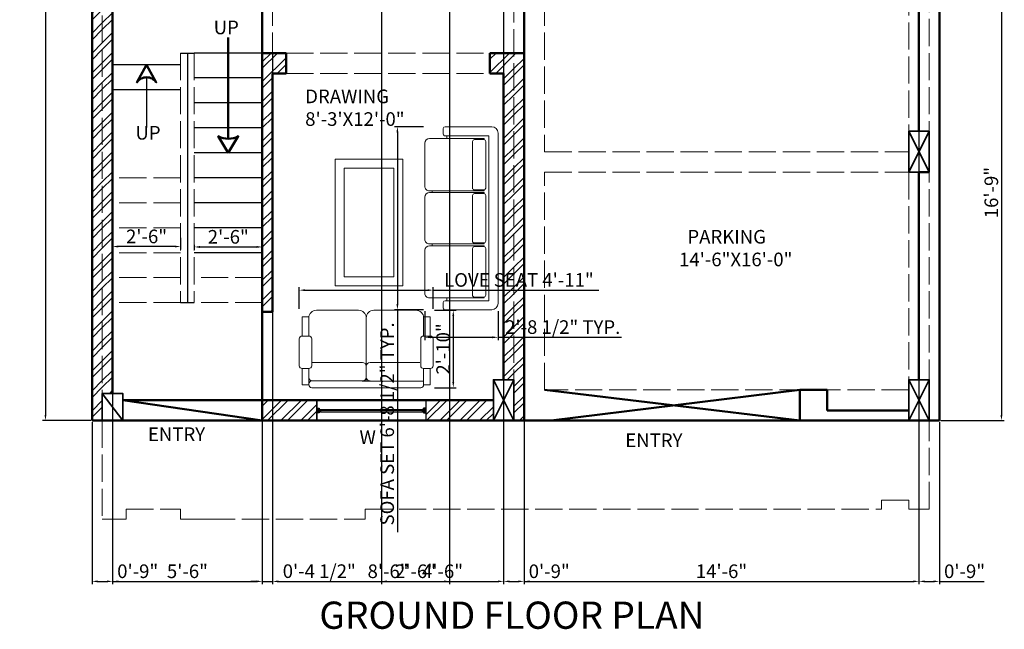
# Model space of a CAD drawing. Units: millimetres. Extents: x 4237 to 5109, y 21391 to 22486.
# Tile 6 of 17: x 4240 to 4674, y 21941 to 22209. Entities that reach past the tile are written whole.
import ezdxf

# ---------------------------------------------------------------- set-up
doc = ezdxf.new("R2010")
doc.units = ezdxf.units.MM
doc.linetypes.add('ACAD_ISO02W100', pattern=[15, 12, -3])
for name, color, linetype, lineweight in [('A-ANNO-DIMS', 2, 'Continuous', 18), ('A-ANNO-TEXT', 7, 'Continuous', 18), ('A-AREA-IDEN', 3, 'Continuous', 18), ('A-FLOR-OVHD', 1, 'ACAD_ISO02W100', 18), ('A-FLOR-STRS', 7, 'Continuous', 25), ('A-FURN', 8, 'Continuous', 18), ('A-WALL', 7, 'Continuous', 50), ('A-WALL-PATT', 252, 'Continuous', 13), ('column', 102, 'Continuous', 35), ('windows', 140, 'Continuous', 25)]:
    doc.layers.add(name, color=color, linetype=linetype, lineweight=lineweight)
doc.styles.get("Standard").update_dxf_attribs({"font": 'arial.ttf'})
doc.dimstyles.new('ISO-25', dxfattribs={"dimtxt": 6, "dimasz": 2.5, "dimexe": 1.25, "dimexo": 0.625, "dimtad": 1, "dimdec": 1, "dimlunit": 4, "dimtxsty": 'Standard', "dimcen": 2.5, "dimadec": 0, "dimazin": 0, "dimtfac": 1, "dimtdec": 1, "dimtmove": 0, "dimatfit": 3, "dimfxl": 1, "dimarcsym": 0})

# ---------------------------------------------------------------- blocks, each defined once
blk = doc.blocks.new('A$C06FC73D7')
for p, q in [((1.93, 0.8), (0.07, 0.8)), ((0, 0.73), (0, 0.22)), ((0.1, 0.22), (0.1, 0.7)), ((0.1, 0.7), (1.9, 0.7)), ((0.13, 0.648), (0.13, 0.05)), ((0.14, 0.648), (0.13, 0.648)), ((0.67, 0.664), (0.16, 0.664)), ((0.7, 0.648), (0.69, 0.648)), ((0.7, 0.05), (0.7, 0.648)), ((0.72, 0.05), (0.72, 0.648)), ((0.73, 0.648), (0.72, 0.648)), ((1.25, 0.664), (0.75, 0.664)), ((1.28, 0.648), (1.27, 0.648)), ((1.28, 0.05), (1.28, 0.648)), ((1.3, 0.05), (1.3, 0.648)), ((1.31, 0.648), (1.3, 0.648)), ((1.84, 0.664), (1.33, 0.664)), ((1.87, 0.648), (1.86, 0.648)), ((1.87, 0.05), (1.87, 0.648)), ((1.9, 0.7), (1.9, 0.22)), ((2, 0.22), (2, 0.73)), ((0.14, 0.54), (0.14, 0.644)), ((0.69, 0.54), (0.69, 0.644)), ((0.73, 0.54), (0.73, 0.644)), ((1.27, 0.54), (1.27, 0.644)), ((1.31, 0.54), (1.31, 0.644)), ((1.86, 0.54), (1.86, 0.644)), ((0.67, 0.52), (0.16, 0.52)), ((1.25, 0.52), (0.75, 0.52)), ((1.84, 0.52), (1.33, 0.52)), ((0.13, 0.24), (0.1, 0.24)), ((1.9, 0.24), (1.87, 0.24)), ((0.02, 0.2), (0.08, 0.2)), ((1.92, 0.2), (1.98, 0.2)), ((0.65, 0), (0.18, 0)), ((0.72, 0.08), (0.7, 0.08)), ((1.23, 0), (0.77, 0)), ((1.3, 0.08), (1.28, 0.08)), ((1.82, 0), (1.35, 0))]:
    blk.add_line(p, q)
for centre, radius, start, end in [((0.07, 0.73), 0.07, 90, 180), ((1.93, 0.73), 0.07, 0, 90), ((0.16, 0.644), 0.02, 90, 180), ((0.67, 0.644), 0.02, 0, 90), ((0.75, 0.644), 0.02, 90, 180), ((1.25, 0.644), 0.02, 0, 90), ((1.33, 0.644), 0.02, 90, 180), ((1.84, 0.644), 0.02, 0, 90), ((0.16, 0.54), 0.02, 180, 270), ((0.67, 0.54), 0.02, 270, 0), ((0.75, 0.54), 0.02, 180, 270), ((1.25, 0.54), 0.02, 270, 0), ((1.33, 0.54), 0.02, 180, 270), ((1.84, 0.54), 0.02, 270, 0), ((0.02, 0.22), 0.02, 180, 270), ((0.08, 0.22), 0.02, 270, 0), ((1.92, 0.22), 0.02, 180, 270), ((1.98, 0.22), 0.02, 270, 0), ((0.18, 0.05), 0.05, 180, 270), ((0.65, 0.05), 0.05, 270, 0), ((0.77, 0.05), 0.05, 180, 270), ((1.23, 0.05), 0.05, 270, 0), ((1.35, 0.05), 0.05, 180, 270), ((1.82, 0.05), 0.05, 270, 0)]:
    blk.add_arc(centre, radius, start, end)
blk = doc.blocks.new('F20')
for p, q in [((-0.558, 0.019), (0.582, 0.019)), ((-0.658, -0.181), (-0.658, -0.011)), ((-0.658, -0.011), (-0.588, -0.011)), ((-0.588, -0.011), (-0.588, -0.021)), ((-0.588, -0.091), (-0.588, -0.011)), ((-0.588, -0.181), (-0.588, -0.091)), ((-0.028, -0.051), (-0.548, -0.051)), ((-0.029, -0.05), (0.06, -0.05)), ((0.012, -0.606), (0.012, -0.051)), ((0.012, -0.205), (0.012, -0.091)), ((0.06, -0.05), (0.612, -0.05)), ((0.612, -0.181), (0.612, -0.01)), ((0.612, -0.011), (0.612, -0.02)), ((0.682, -0.011), (0.612, -0.011)), ((0.612, -0.177), (0.612, -0.08)), ((0.682, -0.181), (0.682, -0.011)), ((-0.658, -0.181), (-0.588, -0.181)), ((0.012, -0.321), (0.012, -0.174)), ((0.682, -0.181), (0.612, -0.181)), ((-0.688, -0.211), (-0.688, -0.491)), ((-0.558, -0.211), (-0.558, -0.491)), ((-0.556, -0.245), (-0.028, -0.245)), ((0.012, -0.285), (0.012, -0.641)), ((0.052, -0.245), (0.572, -0.245)), ((0.582, -0.211), (0.582, -0.491)), ((0.712, -0.211), (0.712, -0.491)), ((-0.658, -0.721), (-0.658, -0.521)), ((-0.658, -0.521), (-0.588, -0.521)), ((-0.588, -0.521), (-0.588, -0.691)), ((0.012, -0.606), (0.012, -0.711)), ((0.612, -0.521), (0.612, -0.691)), ((0.682, -0.521), (0.612, -0.521)), ((0.612, -0.606), (0.612, -0.711)), ((0.612, -0.606), (0.612, -0.711)), ((0.682, -0.721), (0.682, -0.521)), ((-0.588, -0.691), (-0.588, -0.65)), ((-0.588, -0.691), (-0.588, -0.711)), ((0.612, -0.691), (0.612, -0.65)), ((0.612, -0.691), (0.612, -0.711)), ((-0.618, -0.721), (-0.658, -0.721)), ((-0.618, -0.721), (-0.588, -0.721)), ((-0.508, -0.791), (-0.068, -0.791)), ((0.092, -0.791), (0.532, -0.791)), ((0.246, -0.791), (0.246, -0.791)), ((0.642, -0.721), (0.612, -0.721)), ((0.642, -0.721), (0.682, -0.721))]:
    blk.add_line(p, q)
for centre, radius, start, end in [((-0.558, -0.011), 0.03, 90, 180), ((0.582, -0.011), 0.03, 360, 90), ((-0.558, -0.021), 0.03, 180, 270), ((-0.548, -0.091), 0.04, 90, 180), ((-0.028, -0.091), 0.04, 0, 90), ((0.052, -0.091), 0.04, 90, 180), ((-0.658, -0.211), 0.03, 90, 180), ((-0.588, -0.211), 0.03, 0, 90), ((-0.028, -0.205), 0.04, 270, 360), ((0.052, -0.205), 0.04, 180, 270), ((0.612, -0.211), 0.03, 90, 180), ((0.682, -0.211), 0.03, 0, 90), ((-0.658, -0.491), 0.03, 180, 270), ((-0.588, -0.491), 0.03, 270, 360), ((0.612, -0.491), 0.03, 180, 270), ((0.682, -0.491), 0.03, 270, 360), ((-0.508, -0.711), 0.08, 180, 270), ((-0.068, -0.711), 0.08, 270, 360), ((0.092, -0.711), 0.08, 180, 270), ((0.532, -0.711), 0.08, 270, 360)]:
    blk.add_arc(centre, radius, start, end)
blk = doc.blocks.new('*D54')
at = {"layer": 'A-ANNO-DIMS', "color": 0, "lineweight": -2, "transparency": 16777216}
for p, q in [((4280.65, 22113.25), (4280.65, 22108.16)), ((4310.65, 22113.25), (4310.65, 22108.16)), ((4308.15, 22109.41), (4283.15, 22109.41))]:
    blk.add_line(p, q, dxfattribs=at)
at = {"layer": 'A-ANNO-DIMS', "color": 0, "transparency": 16777216}
for points in [[(4283.15, 22109.83), (4283.15, 22109), (4280.65, 22109.41)], [(4308.15, 22109.83), (4308.15, 22109), (4310.65, 22109.41)]]:
    blk.add_solid(points, dxfattribs=at)
at = {"layer": 'Defpoints', "color": 0, "transparency": 16777216}
for p in [(4280.65, 22113.87), (4310.65, 22113.87), (4280.65, 22109.41)]:
    blk.add_point(p, dxfattribs=at)
at = {"layer": 'A-ANNO-DIMS', "color": 0, "transparency": 16777216, "insert": (4295.65, 22113.1), "char_height": 6, "attachment_point": 5}
blk.add_mtext('2\'-6"', dxfattribs=at)
blk = doc.blocks.new('*D55')
at = {"layer": 'A-ANNO-DIMS', "color": 0, "lineweight": -2, "transparency": 16777216}
for p, q in [((4316.65, 22110.15), (4316.65, 22107.98)), ((4319.15, 22109.23), (4344.15, 22109.23)), ((4346.65, 22110.15), (4346.65, 22107.98))]:
    blk.add_line(p, q, dxfattribs=at)
at = {"layer": 'A-ANNO-DIMS', "color": 0, "transparency": 16777216}
for points in [[(4319.15, 22109.65), (4319.15, 22108.81), (4316.65, 22109.23)], [(4344.15, 22109.65), (4344.15, 22108.81), (4346.65, 22109.23)]]:
    blk.add_solid(points, dxfattribs=at)
at = {"layer": 'Defpoints', "color": 0, "transparency": 16777216}
for p in [(4316.65, 22110.78), (4346.65, 22110.78), (4346.65, 22109.23)]:
    blk.add_point(p, dxfattribs=at)
at = {"layer": 'A-ANNO-DIMS', "color": 0, "transparency": 16777216, "insert": (4331.65, 22112.92), "char_height": 6, "attachment_point": 5}
blk.add_mtext('2\'-6"', dxfattribs=at)
blk = doc.blocks.new('*D58')
at = {"layer": 'A-ANNO-DIMS', "color": 0, "lineweight": -2, "transparency": 16777216}
for p, q in [((4271.03, 22440.7), (4249.86, 22440.7)), ((4251.11, 22438.2), (4251.11, 22035.2)), ((4271.03, 22032.7), (4249.86, 22032.7))]:
    blk.add_line(p, q, dxfattribs=at)
at = {"layer": 'A-ANNO-DIMS', "color": 0, "transparency": 16777216}
for points in [[(4250.69, 22438.2), (4251.53, 22438.2), (4251.11, 22440.7)], [(4250.69, 22035.2), (4251.53, 22035.2), (4251.11, 22032.7)]]:
    blk.add_solid(points, dxfattribs=at)
at = {"layer": 'Defpoints', "color": 0, "transparency": 16777216}
for p in [(4271.65, 22440.7), (4251.11, 22032.7), (4271.65, 22032.7)]:
    blk.add_point(p, dxfattribs=at)
at = {"layer": 'A-ANNO-DIMS', "color": 0, "transparency": 16777216, "insert": (4245.89, 22236.7), "char_height": 9, "attachment_point": 5, "rotation": 90}
blk.add_mtext("34'", dxfattribs=at)
blk = doc.blocks.new('*D94')
at = {"layer": 'A-ANNO-DIMS', "color": 0, "lineweight": -2, "transparency": 16777216}
for p, q in [((4417.64, 22162.23), (4404.91, 22162.23)), ((4406.16, 22159.73), (4406.16, 22084.02)), ((4417.64, 22081.52), (4404.91, 22081.52)), ((4406.16, 22081.52), (4406.16, 21983.47))]:
    blk.add_line(p, q, dxfattribs=at)
at = {"layer": 'A-ANNO-DIMS', "color": 0, "transparency": 16777216}
for points in [[(4405.75, 22159.73), (4406.58, 22159.73), (4406.16, 22162.23)], [(4405.75, 22084.02), (4406.58, 22084.02), (4406.16, 22081.52)]]:
    blk.add_solid(points, dxfattribs=at)
at = {"layer": 'Defpoints', "color": 0, "transparency": 16777216}
for p in [(4418.27, 22162.23), (4406.16, 22081.52), (4418.27, 22081.52)]:
    blk.add_point(p, dxfattribs=at)
at = {"layer": 'A-ANNO-DIMS', "color": 0, "transparency": 16777216, "insert": (4402.43, 22031.25), "char_height": 6, "attachment_point": 5, "rotation": 90}
blk.add_mtext('SOFA SET 6\'-8 1/2" TYP.', dxfattribs=at)
blk = doc.blocks.new('*D95')
at = {"layer": 'A-ANNO-DIMS', "color": 0, "lineweight": -2, "transparency": 16777216}
for p, q in [((4418.27, 22080.9), (4418.27, 22068.17)), ((4450.55, 22080.9), (4450.55, 22068.17)), ((4420.77, 22069.42), (4448.05, 22069.42)), ((4450.55, 22069.42), (4504.96, 22069.42))]:
    blk.add_line(p, q, dxfattribs=at)
at = {"layer": 'A-ANNO-DIMS', "color": 0, "transparency": 16777216}
for points in [[(4420.77, 22069.83), (4420.77, 22069), (4418.27, 22069.42)], [(4448.05, 22069.83), (4448.05, 22069), (4450.55, 22069.42)]]:
    blk.add_solid(points, dxfattribs=at)
at = {"layer": 'Defpoints', "color": 0, "transparency": 16777216}
for p in [(4418.27, 22081.52), (4450.55, 22081.52), (4450.55, 22069.42)]:
    blk.add_point(p, dxfattribs=at)
at = {"layer": 'A-ANNO-DIMS', "color": 0, "transparency": 16777216, "insert": (4479, 22073.14), "char_height": 6, "attachment_point": 5}
blk.add_mtext('2\'-8 1/2" TYP.', dxfattribs=at)
blk = doc.blocks.new('*D96')
at = {"layer": 'A-ANNO-DIMS', "color": 0, "lineweight": -2, "transparency": 16777216}
for p, q in [((4362.94, 22081.97), (4362.94, 22091.44)), ((4365.44, 22090.19), (4419.43, 22090.19)), ((4421.93, 22081.97), (4421.93, 22091.44)), ((4421.93, 22090.19), (4494.94, 22090.19))]:
    blk.add_line(p, q, dxfattribs=at)
at = {"layer": 'A-ANNO-DIMS', "color": 0, "transparency": 16777216}
for points in [[(4365.44, 22090.61), (4365.44, 22089.77), (4362.94, 22090.19)], [(4419.43, 22090.61), (4419.43, 22089.77), (4421.93, 22090.19)]]:
    blk.add_solid(points, dxfattribs=at)
at = {"layer": 'Defpoints', "color": 0, "transparency": 16777216}
for p in [(4421.93, 22090.19), (4362.94, 22081.34), (4421.93, 22081.34)]:
    blk.add_point(p, dxfattribs=at)
at = {"layer": 'A-ANNO-DIMS', "color": 0, "transparency": 16777216, "insert": (4459.69, 22093.92), "char_height": 6, "attachment_point": 5}
blk.add_mtext('LOVE SEAT 4\'-11"', dxfattribs=at)
blk = doc.blocks.new('*D97')
at = {"layer": 'A-ANNO-DIMS', "color": 0, "lineweight": -2, "transparency": 16777216}
for p, q in [((4422.56, 22081.34), (4432.03, 22081.34)), ((4430.78, 22078.84), (4430.78, 22049.71)), ((4422.56, 22047.21), (4432.03, 22047.21))]:
    blk.add_line(p, q, dxfattribs=at)
at = {"layer": 'A-ANNO-DIMS', "color": 0, "transparency": 16777216}
for points in [[(4430.36, 22078.84), (4431.2, 22078.84), (4430.78, 22081.34)], [(4430.36, 22049.71), (4431.2, 22049.71), (4430.78, 22047.21)]]:
    blk.add_solid(points, dxfattribs=at)
at = {"layer": 'Defpoints', "color": 0, "transparency": 16777216}
for p in [(4421.93, 22081.34), (4421.93, 22047.21), (4430.78, 22047.21)]:
    blk.add_point(p, dxfattribs=at)
at = {"layer": 'A-ANNO-DIMS', "color": 0, "transparency": 16777216, "insert": (4427.09, 22064.28), "char_height": 6, "attachment_point": 5, "rotation": 90}
blk.add_mtext('2\'-10"', dxfattribs=at)
blk = doc.blocks.new('*D98')
at = {"layer": 'A-ANNO-DIMS', "color": 0, "lineweight": -2, "transparency": 16777216}
for p, q in [((4280.65, 22233.08), (4280.65, 21960.6)), ((4271.65, 22032.08), (4271.65, 21960.6)), ((4274.15, 21961.85), (4278.15, 21961.85)), ((4280.65, 21961.85), (4300.35, 21961.85))]:
    blk.add_line(p, q, dxfattribs=at)
at = {"layer": 'A-ANNO-DIMS', "color": 0, "transparency": 16777216}
for points in [[(4274.15, 21962.27), (4274.15, 21961.43), (4271.65, 21961.85)], [(4278.15, 21962.27), (4278.15, 21961.43), (4280.65, 21961.85)]]:
    blk.add_solid(points, dxfattribs=at)
at = {"layer": 'Defpoints', "color": 0, "transparency": 16777216}
for p in [(4280.65, 22233.7), (4271.65, 22032.7), (4280.65, 21961.85)]:
    blk.add_point(p, dxfattribs=at)
at = {"layer": 'A-ANNO-DIMS', "color": 0, "transparency": 16777216, "insert": (4291.75, 21965.54), "char_height": 6, "attachment_point": 5}
blk.add_mtext('0\'-9"', dxfattribs=at)
blk = doc.blocks.new('*D99')
at = {"layer": 'A-ANNO-DIMS', "color": 0, "lineweight": -2, "transparency": 16777216}
for p, q in [((4280.65, 22233.08), (4280.65, 21960.6)), ((4346.65, 22233.08), (4346.65, 21960.6)), ((4283.15, 21961.85), (4344.15, 21961.85))]:
    blk.add_line(p, q, dxfattribs=at)
at = {"layer": 'A-ANNO-DIMS', "color": 0, "transparency": 16777216}
for points in [[(4283.15, 21962.27), (4283.15, 21961.43), (4280.65, 21961.85)], [(4344.15, 21962.27), (4344.15, 21961.43), (4346.65, 21961.85)]]:
    blk.add_solid(points, dxfattribs=at)
at = {"layer": 'Defpoints', "color": 0, "transparency": 16777216}
for p in [(4280.65, 22233.7), (4346.65, 22233.7), (4346.65, 21961.85)]:
    blk.add_point(p, dxfattribs=at)
at = {"layer": 'A-ANNO-DIMS', "color": 0, "transparency": 16777216, "insert": (4313.65, 21965.54), "char_height": 6, "attachment_point": 5}
blk.add_mtext('5\'-6"', dxfattribs=at)
blk = doc.blocks.new('*D100')
at = {"layer": 'A-ANNO-DIMS', "color": 0, "lineweight": -2, "transparency": 16777216}
for p, q in [((4346.65, 22233.08), (4346.65, 21960.6)), ((4351.15, 22194.08), (4351.15, 21960.6)), ((4344.15, 21961.85), (4341.65, 21961.85)), ((4346.65, 21961.85), (4351.15, 21961.85)), ((4353.65, 21961.85), (4387.33, 21961.85))]:
    blk.add_line(p, q, dxfattribs=at)
at = {"layer": 'A-ANNO-DIMS', "color": 0, "transparency": 16777216}
for points in [[(4344.15, 21962.27), (4344.15, 21961.43), (4346.65, 21961.85)], [(4353.65, 21962.27), (4353.65, 21961.43), (4351.15, 21961.85)]]:
    blk.add_solid(points, dxfattribs=at)
at = {"layer": 'Defpoints', "color": 0, "transparency": 16777216}
for p in [(4346.65, 22233.7), (4351.15, 22194.7), (4351.15, 21961.85)]:
    blk.add_point(p, dxfattribs=at)
at = {"layer": 'A-ANNO-DIMS', "color": 0, "transparency": 16777216, "insert": (4371.74, 21965.58), "char_height": 6, "attachment_point": 5}
blk.add_mtext('0\'-4 1/2"', dxfattribs=at)
blk = doc.blocks.new('*D101')
at = {"layer": 'A-ANNO-DIMS', "color": 0, "lineweight": -2, "transparency": 16777216}
for p, q in [((4351.15, 22194.08), (4351.15, 21960.6)), ((4452.95, 22185.08), (4452.95, 21960.6)), ((4353.65, 21961.85), (4450.45, 21961.85))]:
    blk.add_line(p, q, dxfattribs=at)
at = {"layer": 'A-ANNO-DIMS', "color": 0, "transparency": 16777216}
for points in [[(4353.65, 21962.27), (4353.65, 21961.43), (4351.15, 21961.85)], [(4450.45, 21962.27), (4450.45, 21961.43), (4452.95, 21961.85)]]:
    blk.add_solid(points, dxfattribs=at)
at = {"layer": 'Defpoints', "color": 0, "transparency": 16777216}
for p in [(4351.15, 22194.7), (4452.95, 22185.7), (4452.95, 21961.85)]:
    blk.add_point(p, dxfattribs=at)
at = {"layer": 'A-ANNO-DIMS', "color": 0, "transparency": 16777216, "insert": (4402.05, 21965.54), "char_height": 6, "attachment_point": 5}
blk.add_mtext('8\'-6"', dxfattribs=at)
blk = doc.blocks.new('*D102')
at = {"layer": 'A-ANNO-DIMS', "color": 0, "lineweight": -2, "transparency": 16777216}
for p, q in [((4461.95, 22233.08), (4461.95, 21960.6)), ((4452.95, 22185.08), (4452.95, 21960.6)), ((4455.45, 21961.85), (4459.45, 21961.85)), ((4461.95, 21961.85), (4481.65, 21961.85))]:
    blk.add_line(p, q, dxfattribs=at)
at = {"layer": 'A-ANNO-DIMS', "color": 0, "transparency": 16777216}
for points in [[(4455.45, 21962.27), (4455.45, 21961.43), (4452.95, 21961.85)], [(4459.45, 21962.27), (4459.45, 21961.43), (4461.95, 21961.85)]]:
    blk.add_solid(points, dxfattribs=at)
at = {"layer": 'Defpoints', "color": 0, "transparency": 16777216}
for p in [(4461.95, 22233.7), (4452.95, 22185.7), (4461.95, 21961.85)]:
    blk.add_point(p, dxfattribs=at)
at = {"layer": 'A-ANNO-DIMS', "color": 0, "transparency": 16777216, "insert": (4473.05, 21965.54), "char_height": 6, "attachment_point": 5}
blk.add_mtext('0\'-9"', dxfattribs=at)
blk = doc.blocks.new('*D103')
at = {"layer": 'A-ANNO-DIMS', "color": 0, "lineweight": -2, "transparency": 16777216}
for p, q in [((4461.95, 22233.08), (4461.95, 21960.6)), ((4635.95, 22233.08), (4635.95, 21960.6)), ((4464.45, 21961.85), (4633.45, 21961.85))]:
    blk.add_line(p, q, dxfattribs=at)
at = {"layer": 'A-ANNO-DIMS', "color": 0, "transparency": 16777216}
for points in [[(4464.45, 21962.27), (4464.45, 21961.43), (4461.95, 21961.85)], [(4633.45, 21962.27), (4633.45, 21961.43), (4635.95, 21961.85)]]:
    blk.add_solid(points, dxfattribs=at)
at = {"layer": 'Defpoints', "color": 0, "transparency": 16777216}
for p in [(4461.95, 22233.7), (4635.95, 22233.7), (4635.95, 21961.85)]:
    blk.add_point(p, dxfattribs=at)
at = {"layer": 'A-ANNO-DIMS', "color": 0, "transparency": 16777216, "insert": (4548.95, 21965.54), "char_height": 6, "attachment_point": 5}
blk.add_mtext('14\'-6"', dxfattribs=at)
blk = doc.blocks.new('*D104')
at = {"layer": 'A-ANNO-DIMS', "color": 0, "lineweight": -2, "transparency": 16777216}
for p, q in [((4635.95, 22233.08), (4635.95, 21960.6)), ((4644.95, 22032.08), (4644.95, 21960.6)), ((4638.45, 21961.85), (4642.45, 21961.85)), ((4644.95, 21961.85), (4664.65, 21961.85))]:
    blk.add_line(p, q, dxfattribs=at)
at = {"layer": 'A-ANNO-DIMS', "color": 0, "transparency": 16777216}
for points in [[(4638.45, 21962.27), (4638.45, 21961.43), (4635.95, 21961.85)], [(4642.45, 21962.27), (4642.45, 21961.43), (4644.95, 21961.85)]]:
    blk.add_solid(points, dxfattribs=at)
at = {"layer": 'Defpoints', "color": 0, "transparency": 16777216}
for p in [(4635.95, 22233.7), (4644.95, 22032.7), (4644.95, 21961.85)]:
    blk.add_point(p, dxfattribs=at)
at = {"layer": 'A-ANNO-DIMS', "color": 0, "transparency": 16777216, "insert": (4656.05, 21965.54), "char_height": 6, "attachment_point": 5}
blk.add_mtext('0\'-9"', dxfattribs=at)
blk = doc.blocks.new('*D107')
at = {"layer": 'A-ANNO-DIMS', "color": 0, "lineweight": -2, "transparency": 16777216}
for p, q in [((4636.58, 22233.7), (4673.55, 22233.7)), ((4672.3, 22231.2), (4672.3, 22035.2)), ((4645.58, 22032.7), (4673.55, 22032.7))]:
    blk.add_line(p, q, dxfattribs=at)
at = {"layer": 'A-ANNO-DIMS', "color": 0, "transparency": 16777216}
for points in [[(4671.88, 22231.2), (4672.72, 22231.2), (4672.3, 22233.7)], [(4671.88, 22035.2), (4672.72, 22035.2), (4672.3, 22032.7)]]:
    blk.add_solid(points, dxfattribs=at)
at = {"layer": 'Defpoints', "color": 0, "transparency": 16777216}
for p in [(4635.95, 22233.7), (4644.95, 22032.7), (4672.3, 22032.7)]:
    blk.add_point(p, dxfattribs=at)
at = {"layer": 'A-ANNO-DIMS', "color": 0, "transparency": 16777216, "insert": (4668.61, 22133.2), "char_height": 6, "attachment_point": 5, "rotation": 90}
blk.add_mtext('16\'-9"', dxfattribs=at)
blk = doc.blocks.new('*D110')
at = {"layer": 'A-ANNO-DIMS', "color": 0, "lineweight": -2, "transparency": 16777216}
for p, q in [((4399.15, 22329.08), (4399.15, 21960.6)), ((4452.95, 22329.08), (4452.95, 21960.6)), ((4401.65, 21961.85), (4450.45, 21961.85))]:
    blk.add_line(p, q, dxfattribs=at)
at = {"layer": 'A-ANNO-DIMS', "color": 0, "transparency": 16777216}
for points in [[(4401.65, 21962.27), (4401.65, 21961.43), (4399.15, 21961.85)], [(4450.45, 21962.27), (4450.45, 21961.43), (4452.95, 21961.85)]]:
    blk.add_solid(points, dxfattribs=at)
at = {"layer": 'Defpoints', "color": 0, "transparency": 16777216}
for p in [(4399.15, 22329.7), (4452.95, 22329.7), (4452.95, 21961.85)]:
    blk.add_point(p, dxfattribs=at)
at = {"layer": 'A-ANNO-DIMS', "color": 0, "transparency": 16777216, "insert": (4426.05, 21965.54), "char_height": 6, "attachment_point": 5}
blk.add_mtext('4\'-6"', dxfattribs=at)
blk = doc.blocks.new('*D111')
at = {"layer": 'A-ANNO-DIMS', "color": 0, "lineweight": -2, "transparency": 16777216}
for p, q in [((4399.15, 22324.58), (4399.15, 21960.6)), ((4429.15, 22324.58), (4429.15, 21960.6)), ((4401.65, 21961.85), (4426.65, 21961.85))]:
    blk.add_line(p, q, dxfattribs=at)
at = {"layer": 'A-ANNO-DIMS', "color": 0, "transparency": 16777216}
for points in [[(4401.65, 21962.27), (4401.65, 21961.43), (4399.15, 21961.85)], [(4426.65, 21962.27), (4426.65, 21961.43), (4429.15, 21961.85)]]:
    blk.add_solid(points, dxfattribs=at)
at = {"layer": 'Defpoints', "color": 0, "transparency": 16777216}
for p in [(4399.15, 22325.2), (4429.15, 22325.2), (4429.15, 21961.85)]:
    blk.add_point(p, dxfattribs=at)
at = {"layer": 'A-ANNO-DIMS', "color": 0, "transparency": 16777216, "insert": (4414.15, 21965.54), "char_height": 6, "attachment_point": 5}
blk.add_mtext('2\'-6"', dxfattribs=at)

msp = doc.modelspace()

# ---------------------------------------------------------------- hatches: boundary and pattern name
at = {"layer": 'A-WALL-PATT'}
h = msp.add_hatch(dxfattribs=at)
h.set_pattern_fill('ANSI32', color=256, scale=0.65)
h.paths.add_polyline_path([(4399.15, 22440.7), (4271.65, 22440.7), (4271.65, 22032.7), (4276.15, 22032.7), (4276.15, 22044.7), (4276.15, 22436.2), (4399.15, 22436.2)])
h.paths.add_polyline_path([(4351.15, 22185.7), (4357.15, 22185.7), (4357.15, 22194.7), (4346.65, 22194.7), (4346.65, 22080.7), (4351.15, 22080.7)], flags=16)
h.paths.add_polyline_path([(4351.15, 22295.2), (4346.65, 22295.2), (4346.65, 22238.2), (4311.53, 22238.2), (4311.53, 22233.7), (4351.15, 22233.7)], flags=16)
h = msp.add_hatch(dxfattribs=at)
h.set_pattern_fill('ANSI32', color=256, scale=0.65)
h.paths.add_polyline_path([(4399.15, 22436.2), (4276.15, 22436.2), (4276.15, 22044.7), (4280.65, 22044.7), (4280.65, 22233.7), (4287.73, 22233.7), (4287.73, 22238.2), (4280.65, 22238.2), (4280.65, 22325.2), (4351.15, 22325.2), (4351.15, 22350.7), (4346.65, 22350.7), (4346.65, 22329.7), (4280.65, 22329.7), (4280.65, 22431.7), (4394.65, 22431.7), (4399.15, 22431.7)], flags=17)
h.paths.add_polyline_path([(4351.15, 22185.7), (4357.15, 22185.7), (4357.15, 22194.7), (4346.65, 22194.7), (4346.65, 22080.7), (4351.15, 22080.7)], flags=16)
h.paths.add_polyline_path([(4351.15, 22295.2), (4346.65, 22295.2), (4346.65, 22238.2), (4311.53, 22238.2), (4311.53, 22233.7), (4351.15, 22233.7)], flags=16)
h = msp.add_hatch(dxfattribs=at)
h.set_pattern_fill('ANSI32', color=256, scale=0.65)
h.paths.add_polyline_path([(4457.45, 22194.7), (4446.95, 22194.7), (4446.95, 22185.7), (4452.95, 22185.7), (4452.95, 22050.7), (4457.45, 22050.7)])
h = msp.add_hatch(dxfattribs=at)
h.set_pattern_fill('ANSI32', color=256, scale=0.65)
h.paths.add_polyline_path([(4461.95, 22194.7), (4457.45, 22194.7), (4457.45, 22032.7), (4461.95, 22032.7)])
h = msp.add_hatch(dxfattribs=at)
h.set_pattern_fill('ANSI32', color=256, scale=0.65)
h.paths.add_polyline_path([(4370.65, 22041.7), (4346.65, 22041.7), (4346.65, 22032.7), (4370.65, 22032.7)], flags=17)
h = msp.add_hatch(dxfattribs=at)
h.set_pattern_fill('ANSI32', color=256, scale=0.65)
h.paths.add_polyline_path([(4448.45, 22041.7), (4418.65, 22041.7), (4418.65, 22032.7), (4448.45, 22032.7)])
h = msp.add_hatch(color=256, dxfattribs=at)
h.dxf.hatch_style = 1
h.paths.add_polyline_path([(4372.28, 22037.61), (4371.65, 22037.61), (4371.65, 22038.2), (4370.65, 22038.2), (4370.65, 22036.2), (4371.65, 22036.2), (4371.65, 22036.61), (4372.28, 22036.61)])
h = msp.add_hatch(color=256, dxfattribs=at)
h.dxf.hatch_style = 1
h.paths.add_polyline_path([(4418.65, 22038.2), (4417.65, 22038.2), (4417.65, 22037.61), (4417.03, 22037.61), (4417.03, 22036.61), (4417.65, 22036.61), (4417.65, 22036.2), (4418.65, 22036.2)])

# ---------------------------------------------------------------- linework, layer by layer
at = {"layer": 'A-FLOR-OVHD'}
for p, q in [((4457.45, 22415.2), (4457.45, 22032.7)), ((4351.15, 22233.7), (4351.15, 22194.7)), ((4310.65, 22194.7), (4310.65, 22084.7)), ((4316.65, 22194.7), (4316.65, 22084.7)), ((4357.15, 22194.7), (4446.95, 22194.7)), ((4357.15, 22185.7), (4446.95, 22185.7)), ((4310.65, 22139.7), (4280.65, 22139.7)), ((4310.65, 22128.7), (4280.65, 22128.7)), ((4310.65, 22117.7), (4280.65, 22117.7)), ((4310.65, 22106.7), (4280.65, 22106.7)), ((4310.65, 22095.7), (4280.65, 22095.7)), ((4346.65, 22095.7), (4316.65, 22095.7)), ((4310.65, 22084.7), (4280.65, 22084.7)), ((4346.65, 22084.7), (4316.65, 22084.7))]:
    msp.add_line(p, q, dxfattribs=at)
for points in [[(4640.45, 22032.7), (4640.45, 22436.2), (4276.15, 22436.2), (4276.15, 22032.7)], [(4470.95, 22233.7), (4470.95, 22151.2), (4631.45, 22151.2), (4631.45, 22233.7)], [(4276.15, 22032.7), (4276.15, 21989.2), (4286.65, 21989.2), (4286.65, 21993.7), (4310.65, 21993.7), (4310.65, 21989.2), (4322.65, 21989.2), (4391.89, 21989.2), (4391.89, 21993.7), (4619.45, 21993.7), (4619.45, 21997.7), (4631.45, 21997.7), (4631.45, 21993.7), (4640.45, 21993.7), (4640.45, 22032.7)]]:
    msp.add_lwpolyline(points, dxfattribs=at)
msp.add_lwpolyline([(4470.95, 22142.2), (4631.45, 22142.2), (4631.45, 22046.2), (4470.95, 22046.2)], close=True, dxfattribs=at)
at = {"layer": 'A-FLOR-STRS'}
for p, q in [((4310.65, 22194.7), (4316.65, 22194.7)), ((4313.65, 22194.7), (4313.65, 22084.7)), ((4346.65, 22194.7), (4316.65, 22194.7)), ((4310.65, 22189.54), (4280.65, 22189.54)), ((4295.65, 22184.01), (4295.65, 22161.83)), ((4346.65, 22183.7), (4316.65, 22183.7)), ((4310.65, 22178.54), (4280.65, 22178.54)), ((4346.65, 22172.7), (4316.65, 22172.7)), ((4346.65, 22161.7), (4316.65, 22161.7)), ((4346.65, 22150.7), (4316.65, 22150.7)), ((4346.65, 22139.7), (4316.65, 22139.7)), ((4346.65, 22128.7), (4316.65, 22128.7)), ((4346.65, 22117.7), (4316.65, 22117.7)), ((4346.65, 22106.7), (4316.65, 22106.7)), ((4310.65, 22084.7), (4316.65, 22084.7))]:
    msp.add_line(p, q, dxfattribs=at)
at = {"layer": 'A-FURN'}
for points in [[(4378.77, 22147.95), (4408.57, 22147.95), (4408.57, 22092.07), (4378.77, 22092.07)], [(4382.77, 22143.95), (4404.57, 22143.95), (4404.57, 22096.07), (4382.77, 22096.07)]]:
    msp.add_lwpolyline(points, close=True, dxfattribs=at)
at = {"layer": 'A-WALL'}
for p, q in [((4271.65, 22440.7), (4271.65, 22032.7)), ((4644.95, 22440.7), (4644.95, 22032.7)), ((4280.65, 22233.7), (4280.65, 22044.7)), ((4346.65, 22194.7), (4346.65, 22233.7)), ((4461.95, 22233.7), (4461.95, 22194.7)), ((4635.95, 22233.7), (4635.95, 22160.2)), ((4331.65, 22156.91), (4331.65, 22201.56)), ((4346.65, 22194.7), (4357.15, 22194.7)), ((4346.65, 22194.7), (4346.65, 22080.7)), ((4357.15, 22194.7), (4357.15, 22185.7)), ((4446.95, 22194.7), (4446.95, 22185.7)), ((4446.95, 22194.7), (4461.95, 22194.7)), ((4461.95, 22194.7), (4461.95, 22032.7)), ((4351.15, 22185.7), (4357.15, 22185.7)), ((4351.15, 22185.7), (4351.15, 22080.7)), ((4446.95, 22185.7), (4452.95, 22185.7)), ((4452.95, 22185.7), (4452.95, 22050.7)), ((4635.95, 22142.2), (4640.45, 22142.2)), ((4635.95, 22142.2), (4635.95, 22050.7)), ((4346.65, 22080.7), (4351.15, 22080.7)), ((4346.65, 22080.7), (4346.65, 22032.7)), ((4470.95, 22046.2), (4583.45, 22032.7)), ((4583.45, 22046.2), (4473.95, 22032.7)), ((4583.45, 22046.2), (4595.45, 22046.2)), ((4346.65, 22041.7), (4285.15, 22041.7)), ((4285.15, 22041.7), (4346.65, 22032.7)), ((4448.45, 22041.7), (4346.65, 22041.7)), ((4595.45, 22037.2), (4631.45, 22037.2)), ((4271.65, 22032.7), (4285.15, 22032.7)), ((4285.15, 22032.7), (4346.65, 22032.7)), ((4346.65, 22032.7), (4448.45, 22032.7)), ((4346.65, 22032.7), (4644.95, 22032.7))]:
    msp.add_line(p, q, dxfattribs=at)
for points in [[(4295.65, 22189.54), (4299.91, 22181.74, 0.534219), (4291.39, 22181.74)], [(4331.65, 22150.7), (4336.04, 22157.99, -0.245903), (4327.26, 22157.99)]]:
    msp.add_lwpolyline(points, format="xyb", close=True, dxfattribs=at)
for points in [[(4583.45, 22032.7), (4583.45, 22046.2)], [(4595.45, 22037.2), (4595.45, 22046.2)]]:
    msp.add_lwpolyline(points, dxfattribs=at)
at = {"layer": 'column'}
for p, q in [((4631.45, 22160.2), (4640.45, 22142.2)), ((4640.45, 22160.2), (4631.45, 22142.2)), ((4448.45, 22050.7), (4457.45, 22032.7)), ((4448.45, 22032.7), (4457.45, 22050.7)), ((4640.45, 22050.7), (4631.45, 22032.7)), ((4640.45, 22032.7), (4631.45, 22050.7)), ((4276.15, 22044.7), (4276.15, 22032.7)), ((4276.15, 22044.7), (4285.15, 22032.7))]:
    msp.add_line(p, q, dxfattribs=at)
for points in [[(4640.45, 22142.2), (4631.45, 22142.2), (4631.45, 22160.2), (4640.45, 22160.2)], [(4457.45, 22032.7), (4448.45, 22032.7), (4448.45, 22050.7), (4457.45, 22050.7)], [(4640.45, 22032.7), (4631.45, 22032.7), (4631.45, 22050.7), (4640.45, 22050.7)], [(4276.15, 22032.7), (4285.15, 22032.7), (4285.15, 22044.7), (4276.15, 22044.7)]]:
    msp.add_lwpolyline(points, close=True, dxfattribs=at)
at = {"layer": 'windows'}
for p, q in [((4370.65, 22041.7), (4370.65, 22032.7)), ((4418.65, 22041.7), (4418.65, 22032.7)), ((4372.28, 22037.61), (4372.28, 22036.61)), ((4372.28, 22037.61), (4417.03, 22037.61)), ((4417.03, 22037.11), (4372.28, 22037.11)), ((4417.03, 22037.61), (4417.03, 22036.61)), ((4372.28, 22036.61), (4417.03, 22036.61))]:
    msp.add_line(p, q, dxfattribs=at)
msp.add_lwpolyline([(4370.65, 22041.7), (4418.65, 22041.7), (4418.65, 22032.7), (4370.65, 22032.7)], close=True, dxfattribs=at)
for points in [[(4370.65, 22038.2), (4371.65, 22038.2), (4371.65, 22037.61), (4372.28, 22037.61)], [(4418.65, 22038.2), (4417.65, 22038.2), (4417.65, 22037.61), (4417.03, 22037.61)], [(4372.28, 22036.61), (4371.65, 22036.61), (4371.65, 22036.2), (4370.65, 22036.2)], [(4417.03, 22036.61), (4417.65, 22036.61), (4417.65, 22036.2), (4418.65, 22036.2)]]:
    msp.add_lwpolyline(points, dxfattribs=at)

# ---------------------------------------------------------------- block references
at = {"layer": 'A-FURN'}
for name, p, xscale, yscale, zscale, rotation in [('A$C06FC73D7', (4418.27, 22162.23), 40.35424995786203, 40.35424995786203, 40.35424995786203, 270), ('F20', (4391.92, 22048.02), -42.13697876875379, 42.13697876875379, 42.13697876875379, 180)]:
    msp.add_blockref(name, p, dxfattribs=dict(at, xscale=xscale, yscale=yscale, zscale=zscale, rotation=rotation))

# ---------------------------------------------------------------- texts
at = {"layer": 'A-ANNO-TEXT', "attachment_point": 1}
for s, width, insert, char_height in [('   UP', 21.7253, (4319.71, 22208.97), 6), ('   UP', 21.7253, (4285.24, 22162.54), 6), ('   ENTRY', 72.5927, (4290.75, 22029.71), 6), ('    W', 21.7253, (4382.14, 22028.36), 6), ('   ENTRY', 72.5927, (4501.06, 22027.05), 6), ('    GROUND FLOOR PLAN', 222.3103, (4357.09, 21952.95), 12)]:
    msp.add_mtext_dynamic_manual_height_columns(s, width=width, gutter_width=12.5, heights=[0], dxfattribs=dict(at, insert=insert, char_height=char_height))
at = {"layer": 'A-AREA-IDEN', "char_height": 6, "attachment_point": 1}
for s, insert in [('     DRAWING\\P     8\'-3\'X12\'-0"', (4356.37, 22178.59)), ('   PARKING\\P 14\'-6"X16\'-0"', (4528.43, 22116.72))]:
    msp.add_mtext_dynamic_manual_height_columns(s, width=72.5927, gutter_width=12.5, heights=[0], dxfattribs=dict(at, insert=insert))

# ---------------------------------------------------------------- dimensions: what is measured, and where the dimension line sits
at = {"layer": 'A-ANNO-DIMS'}
for base, p1, p2, angle, override, picture, middle in [((4251.11, 22032.7), (4271.65, 22440.7), (4271.65, 22032.7), 90, {"dimtxt": 9, "dimclrd": 0, "dimclre": 0, "dimclrt": 0}, '*D58', (4245.89, 22236.7)), ((4672.3, 22032.7), (4635.95, 22233.7), (4644.95, 22032.7), 90, {"dimdec": 1, "dimlfac": 1, "dimrnd": 0, "dimzin": 1, "dimdsep": 46, "dimlunit": 4, "dimfrac": 2}, '*D107', (4668.61, 22133.2)), ((4430.78, 22047.21), (4421.93, 22081.34), (4421.93, 22047.21), 270, {"dimdec": 1, "dimrnd": 0, "dimzin": 1, "dimlunit": 4, "dimfrac": 2}, '*D97', (4427.09, 22064.28))]:
    dim = msp.add_linear_dim(base=base, p1=p1, p2=p2, angle=angle, dimstyle='ISO-25', override=override, dxfattribs=at)
    dim.commit()
    dim.dimension.update_dxf_attribs({"geometry": picture, "text_midpoint": middle})
for base, p1, p2, override, picture, middle in [((4452.95, 21961.85), (4399.15, 22329.7), (4452.95, 22329.7), {"dimdec": 1, "dimlfac": 1, "dimrnd": 0, "dimzin": 1, "dimdsep": 46, "dimlunit": 4, "dimfrac": 2}, '*D110', (4426.05, 21965.54)), ((4429.15, 21961.85), (4399.15, 22325.2), (4429.15, 22325.2), {"dimdec": 1, "dimlfac": 1, "dimrnd": 0, "dimzin": 1, "dimdsep": 46, "dimlunit": 4, "dimfrac": 2}, '*D111', (4414.15, 21965.54)), ((4280.65, 21961.85), (4271.65, 22032.7), (4280.65, 22233.7), {"dimdec": 1, "dimlfac": 1, "dimrnd": 0, "dimzin": 1, "dimdsep": 46, "dimlunit": 4, "dimfrac": 2}, '*D98', (4291.75, 21965.54)), ((4346.65, 21961.85), (4280.65, 22233.7), (4346.65, 22233.7), {"dimdec": 1, "dimlfac": 1, "dimrnd": 0, "dimzin": 1, "dimdsep": 46, "dimlunit": 4, "dimfrac": 2}, '*D99', (4313.65, 21965.54)), ((4351.15, 21961.85), (4346.65, 22233.7), (4351.15, 22194.7), {"dimdec": 1, "dimlfac": 1, "dimrnd": 0, "dimzin": 1, "dimdsep": 46, "dimlunit": 4, "dimfrac": 2}, '*D100', (4371.74, 21965.58)), ((4461.95, 21961.85), (4452.95, 22185.7), (4461.95, 22233.7), {"dimdec": 1, "dimlfac": 1, "dimrnd": 0, "dimzin": 1, "dimdsep": 46, "dimlunit": 4, "dimfrac": 2}, '*D102', (4473.05, 21965.54)), ((4635.95, 21961.85), (4461.95, 22233.7), (4635.95, 22233.7), {"dimdec": 1, "dimlfac": 1, "dimrnd": 0, "dimzin": 1, "dimdsep": 46, "dimlunit": 4, "dimfrac": 2}, '*D103', (4548.95, 21965.54)), ((4644.95, 21961.85), (4635.95, 22233.7), (4644.95, 22032.7), {"dimdec": 1, "dimlfac": 1, "dimrnd": 0, "dimzin": 1, "dimdsep": 46, "dimlunit": 4, "dimfrac": 2}, '*D104', (4656.05, 21965.54)), ((4452.95, 21961.85), (4351.15, 22194.7), (4452.95, 22185.7), {"dimdec": 1, "dimlfac": 1, "dimrnd": 0, "dimzin": 1, "dimdsep": 46, "dimlunit": 4, "dimfrac": 2}, '*D101', (4402.05, 21965.54)), ((4280.65, 22109.41), (4310.65, 22113.87), (4280.65, 22113.87), {"dimclrd": 0, "dimclre": 0, "dimclrt": 0}, '*D54', (4295.65, 22113.1)), ((4346.65, 22109.23), (4316.65, 22110.78), (4346.65, 22110.78), {"dimclrd": 0, "dimclre": 0, "dimclrt": 0}, '*D55', (4331.65, 22112.92))]:
    dim = msp.add_linear_dim(base=base, p1=p1, p2=p2, dimstyle='ISO-25', override=override, dxfattribs=at)
    dim.commit()
    dim.dimension.update_dxf_attribs({"geometry": picture, "text_midpoint": middle})
dim = msp.add_linear_dim(base=(4406.16, 22081.52), p1=(4418.27, 22162.23), p2=(4418.27, 22081.52), angle=270, text='SOFA SET <> TYP.', dimstyle='ISO-25', override={"dimdec": 1, "dimrnd": 0, "dimzin": 1, "dimlunit": 4, "dimfrac": 2}, dxfattribs=at)
dim.commit()
dim.dimension.update_dxf_attribs({"geometry": '*D94', "text_midpoint": (4402.43, 22031.25)})
for base, p1, p2, text, picture, middle in [((4421.93, 22090.19), (4362.94, 22081.34), (4421.93, 22081.34), 'LOVE SEAT <>', '*D96', (4459.69, 22093.92)), ((4450.55, 22069.42), (4418.27, 22081.52), (4450.55, 22081.52), '<> TYP.', '*D95', (4479, 22073.14))]:
    dim = msp.add_linear_dim(base=base, p1=p1, p2=p2, text=text, dimstyle='ISO-25', override={"dimdec": 1, "dimrnd": 0, "dimzin": 1, "dimlunit": 4, "dimfrac": 2}, dxfattribs=at)
    dim.commit()
    dim.dimension.update_dxf_attribs({"geometry": picture, "text_midpoint": middle})

doc.saveas('drawing.dxf')
